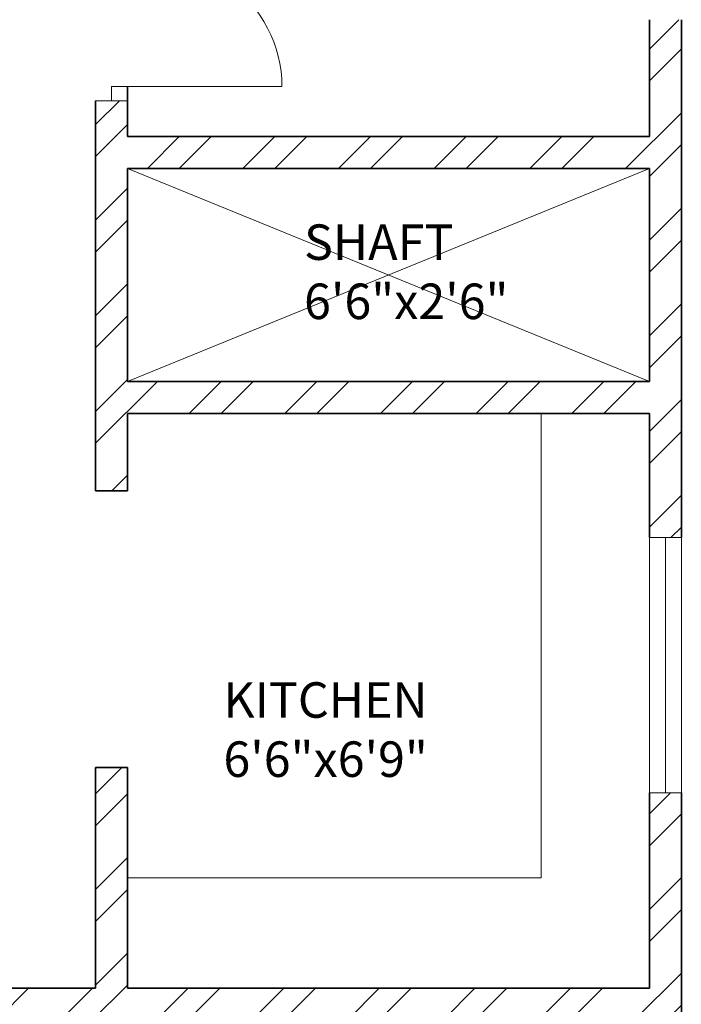
# Model space of a CAD drawing. Units: inches. Extents: x 2168 to 3056, y 1130 to 2629.
# Tile 34 of 42: x 2771 to 2864, y 2079 to 2217. Entities that reach past the tile are written whole.
import ezdxf

# ---------------------------------------------------------------- set-up
doc = ezdxf.new("R2010")
doc.units = ezdxf.units.IN
for name, color, linetype, lineweight in [('A-AREA-IDEN', 7, 'Continuous', 18), ('A-DOOR', 21, 'Continuous', 18), ('A-FLOR-CASE', 71, 'Continuous', 18), ('A-FLOR-OTLN', 7, 'Continuous', 18), ('A-GLAZ', 201, 'Continuous', 18), ('A-WALL', 7, 'Continuous', 35)]:
    doc.layers.add(name, color=color, linetype=linetype, lineweight=lineweight)
doc.layers.add('A-WALL-PATT', color=143, linetype='Continuous', lineweight=13, true_color=0x7aafdf)
doc.styles.get("Standard").update_dxf_attribs({"font": 'arial.ttf'})

msp = doc.modelspace()

# ---------------------------------------------------------------- hatches: boundary and pattern name
at = {"layer": 'A-WALL-PATT'}
h = msp.add_hatch(dxfattribs=at)
h.set_pattern_fill('ANSI32', color=256)
h.paths.add_polyline_path([(2463.8, 2409.39), (2467.39, 2409.39), (2467.39, 2413.89), (2454.77, 2413.89), (2454.77, 2411.64), (2454.77, 2409.39), (2459.3, 2409.39), (2459.3, 2265.39), (2455.64, 2265.39), (2455.64, 2260.89), (2467.35, 2260.89), (2467.35, 2263.14), (2467.35, 2265.39), (2463.8, 2265.39)])
h.paths.add_polyline_path([(2431.6, 2413.89), (2409.65, 2413.89), (2409.65, 2409.39), (2431.6, 2409.39), (2431.6, 2411.64)])
h.paths.add_polyline_path([(2349.65, 2413.89), (2331.8, 2413.89), (2331.8, 2362.67), (2336.3, 2362.67), (2336.3, 2409.39), (2349.65, 2409.39), (2349.65, 2411.64)])
h.paths.add_polyline_path([(2634.15, 2411.64), (2634.15, 2413.89), (2562.29, 2413.89), (2562.29, 2409.39), (2595.8, 2409.39), (2595.8, 2280.31), (2595.83, 2280.31), (2595.83, 2265.39), (2499.91, 2265.39), (2499.91, 2260.89), (2550.8, 2260.89), (2550.8, 2117.31), (2555.3, 2117.31), (2555.3, 2168.08), (2571.93, 2168.08), (2571.93, 2176.89), (2559.8, 2176.89), (2559.8, 2256.39), (2640.8, 2256.39), (2640.8, 2176.89), (2626.43, 2176.89), (2626.43, 2168.08), (2645.3, 2168.08), (2645.3, 2116.64), (2649.8, 2116.64), (2649.8, 2260.89), (2691.25, 2260.89), (2691.25, 2263.14), (2691.25, 2265.39), (2670.65, 2265.39), (2670.65, 2265.36), (2600.3, 2265.36), (2600.3, 2280.26), (2600.3, 2409.39), (2634.15, 2409.39)])
h.paths.add_polyline_path([(2600.3, 2473.89), (2612.84, 2473.89), (2612.84, 2478.39), (2572.64, 2478.39), (2572.64, 2473.89), (2595.8, 2473.89), (2595.8, 2413.89), (2600.3, 2413.89)])
h.paths.add_polyline_path([(2535.8, 2473.89), (2548.64, 2473.89), (2548.64, 2478.39), (2531.4, 2478.39), (2531.4, 2413.89), (2521.6, 2413.89), (2521.6, 2409.39), (2539.24, 2409.39), (2539.24, 2411.64), (2539.24, 2413.89), (2535.8, 2413.89)])
h.paths.add_polyline_path([(2664.8, 2478.39), (2636.84, 2478.39), (2636.84, 2473.89), (2660.3, 2473.89), (2660.3, 2413.89), (2656.17, 2413.89), (2656.17, 2409.39), (2671.68, 2409.39), (2671.68, 2411.64), (2671.68, 2413.89), (2664.8, 2413.89)])
h.paths.add_polyline_path([(2705.94, 2413.89), (2695.68, 2413.89), (2695.68, 2409.39), (2705.94, 2409.39)])
h.paths.add_polyline_path([(2741.35, 2413.89), (2728.73, 2413.89), (2728.73, 2411.64), (2728.73, 2409.39), (2732.3, 2409.39), (2732.3, 2265.39), (2725.73, 2265.39), (2725.73, 2260.89), (2740.92, 2260.89), (2740.92, 2263.14), (2740.92, 2265.39), (2736.8, 2265.39), (2736.8, 2409.39), (2741.35, 2409.39)])
h.paths.add_polyline_path([(2785.65, 2413.89), (2764.55, 2413.89), (2764.49, 2409.39), (2785.65, 2409.39), (2785.65, 2411.64)])
h.paths.add_polyline_path([(2864.3, 2413.89), (2845.65, 2413.89), (2845.65, 2409.39), (2859.8, 2409.39), (2859.8, 2368.43), (2864.3, 2368.43)])
h.paths.add_polyline_path([(2864.3, 2308.43), (2862.05, 2308.43), (2859.8, 2308.43), (2859.8, 2265.39), (2774.48, 2265.39), (2774.48, 2263.14), (2774.48, 2260.89), (2781.8, 2260.89), (2781.8, 2226.65), (2786.3, 2226.65), (2786.3, 2260.89), (2859.8, 2260.89), (2859.8, 2241.35), (2864.3, 2241.35)])
h.paths.add_polyline_path([(2864.3, 2217.35), (2862.05, 2217.35), (2859.8, 2217.35), (2859.8, 2200.89), (2786.3, 2200.89), (2786.3, 2205.93), (2784.05, 2205.93), (2781.8, 2205.93), (2781.8, 2150.97), (2786.3, 2150.97), (2786.3, 2161.89), (2859.8, 2161.89), (2859.8, 2144.42), (2864.3, 2144.42)])
h.paths.add_polyline_path([(2859.8, 2196.39), (2859.8, 2166.39), (2786.3, 2166.39), (2786.3, 2196.39)], flags=16)
h.paths.add_polyline_path([(2864.3, 2108.42), (2862.05, 2108.42), (2859.8, 2108.42), (2859.8, 2080.89), (2786.3, 2080.89), (2786.3, 2111.99), (2781.8, 2111.99), (2781.8, 2080.89), (2649.8, 2080.89), (2649.8, 2086.04), (2647.55, 2086.04), (2645.3, 2086.04), (2645.3, 2071.74), (2649.8, 2071.74), (2649.8, 2076.39), (2781.8, 2076.39), (2781.8, 2041.79), (2786.3, 2041.79), (2786.3, 2076.39), (2859.8, 2076.39), (2859.8, 2058.58), (2864.3, 2058.58)])
h.paths.add_polyline_path([(2864.3, 2022.58), (2859.8, 2022.58), (2859.8, 1992.39), (2786.3, 1992.39), (2786.3, 1999.57), (2781.8, 1999.57), (2781.8, 1848.09), (2784.05, 1848.09), (2786.3, 1848.09), (2786.3, 1851.39), (2859.8, 1851.39), (2859.8, 1838.26), (2864.3, 1838.26)], flags=17)
h.paths.add_polyline_path([(2859.8, 1987.89), (2859.8, 1855.89), (2786.3, 1855.89), (2786.3, 1987.89)], flags=16)
h.paths.add_polyline_path([(2823.05, 1987.89), (2841.42, 1921.89), (2823.05, 1855.89)], flags=0)
h.paths.add_polyline_path([(2864.3, 1814.26), (2859.8, 1814.26), (2859.8, 1791.39), (2786.3, 1791.39), (2786.3, 1825.66), (2784.05, 1825.66), (2781.8, 1825.66), (2781.8, 1791.39), (2720.15, 1791.39), (2720.15, 1791.27), (2649.8, 1791.27), (2649.8, 1806.16), (2649.8, 2038.98), (2647.55, 2038.98), (2645.3, 2038.98), (2645.3, 1783.93), (2649.8, 1783.93), (2649.8, 1786.89), (2781.8, 1786.89), (2781.8, 1746.79), (2786.3, 1746.79), (2786.3, 1786.89), (2859.8, 1786.89), (2859.8, 1770.08), (2864.3, 1770.08)])
h.paths.add_polyline_path([(2864.3, 1734.08), (2862.05, 1734.08), (2859.8, 1734.08), (2859.8, 1705.89), (2786.3, 1705.89), (2786.3, 1714.17), (2781.8, 1714.17), (2781.8, 1660.53), (2786.3, 1660.53), (2786.3, 1666.89), (2859.8, 1666.89), (2859.8, 1648.34), (2864.3, 1648.34)])
h.paths.add_polyline_path([(2786.3, 1701.39), (2859.8, 1701.39), (2859.8, 1671.39), (2786.3, 1671.39)], flags=16)
h.paths.add_polyline_path([(2649.8, 1756.58), (2647.55, 1756.58), (2645.3, 1756.58), (2645.3, 1606.89), (2555.3, 1606.89), (2555.3, 1749.51), (2553.05, 1749.51), (2550.8, 1749.51), (2550.8, 1606.89), (2503.01, 1606.89), (2503.01, 1604.64), (2503.01, 1602.39), (2595.8, 1602.39), (2595.85, 1602.39), (2595.85, 1587.5), (2595.8, 1458.39), (2561.5, 1458.39), (2561.5, 1456.14), (2561.5, 1453.89), (2595.8, 1453.89), (2595.8, 1381.89), (2573.44, 1381.89), (2573.44, 1377.39), (2613.01, 1377.39), (2613.01, 1379.64), (2613.01, 1381.89), (2600.3, 1381.89), (2600.3, 1453.89), (2634.33, 1453.89), (2634.33, 1458.39), (2600.3, 1458.39), (2600.3, 1602.39), (2670.65, 1602.39), (2694.09, 1602.39), (2694.09, 1606.89), (2649.8, 1606.89)])
h.paths.add_polyline_path([(2736.8, 1602.39), (2741.56, 1602.39), (2741.56, 1606.89), (2726.2, 1606.89), (2726.2, 1604.64), (2726.2, 1602.39), (2732.3, 1602.39), (2732.3, 1458.39), (2727.9, 1458.39), (2727.9, 1453.89), (2740.82, 1453.89), (2740.82, 1456.14), (2740.82, 1458.39), (2736.8, 1458.39)])
h.paths.add_polyline_path([(2859.8, 1606.89), (2786.3, 1606.89), (2786.3, 1637.33), (2784.05, 1637.33), (2781.8, 1637.33), (2781.8, 1606.89), (2775.61, 1606.89), (2775.61, 1602.39), (2859.8, 1602.39)])
h.paths.add_polyline_path([(2864.3, 1624.34), (2862.05, 1624.34), (2859.8, 1624.34), (2859.8, 1570.39), (2864.3, 1570.39)])
h.paths.add_polyline_path([(2864.3, 1510.39), (2862.05, 1510.39), (2859.8, 1510.39), (2859.8, 1458.39), (2846.73, 1458.39), (2846.73, 1456.14), (2846.73, 1453.89), (2864.3, 1453.89)])
h.paths.add_polyline_path([(2786.73, 1458.39), (2765.44, 1458.39), (2765.44, 1453.89), (2786.73, 1453.89)])
h.paths.add_polyline_path([(2706, 1458.39), (2695.36, 1458.39), (2695.36, 1453.89), (2706, 1453.89), (2706, 1456.14)])
h.paths.add_polyline_path([(2671.36, 1456.14), (2671.36, 1458.39), (2655.99, 1458.39), (2655.99, 1456.14), (2655.99, 1453.89), (2660.3, 1453.89), (2660.3, 1381.89), (2637.01, 1381.89), (2637.01, 1377.39), (2664.8, 1377.39), (2664.8, 1453.89), (2671.36, 1453.89)], flags=17)
h.paths.add_polyline_path([(2539.83, 1458.39), (2520.24, 1458.39), (2520.24, 1453.89), (2531.3, 1453.89), (2531.3, 1377.39), (2546.45, 1377.39), (2546.45, 1379.64), (2546.45, 1381.89), (2535.8, 1381.89), (2535.8, 1453.89), (2539.83, 1453.89)], flags=17)
h.paths.add_polyline_path([(2496.24, 1458.39), (2489.13, 1458.39), (2489.13, 1453.89), (2496.24, 1453.89), (2496.24, 1456.14)])
h.paths.add_polyline_path([(2467.43, 1456.14), (2467.43, 1458.39), (2463.8, 1458.39), (2463.8, 1602.39), (2468.24, 1602.39), (2468.24, 1605.7), (2468.24, 1606.89), (2454.6, 1606.89), (2454.6, 1602.39), (2459.3, 1602.39), (2459.3, 1458.39), (2454.24, 1458.39), (2454.24, 1453.89), (2467.43, 1453.89)])
h.paths.add_polyline_path([(2431.6, 1456.14), (2431.6, 1458.39), (2411.39, 1458.39), (2411.39, 1453.89), (2431.6, 1453.89)])
h.paths.add_polyline_path([(2351.39, 1458.39), (2336.3, 1458.39), (2336.3, 1490.69), (2334.05, 1490.69), (2331.8, 1490.69), (2331.8, 1453.89), (2351.39, 1453.89), (2351.39, 1456.14)])
h.paths.add_polyline_path([(2336.3, 1629.7), (2331.8, 1629.7), (2331.8, 1552.32), (2336.3, 1552.32), (2336.3, 1602.39), (2406.65, 1602.39), (2423.47, 1602.39), (2423.47, 1606.89), (2418.8, 1606.89), (2418.8, 1643.68), (2416.55, 1643.68), (2414.3, 1643.68), (2414.3, 1606.89), (2336.3, 1606.89)])
h.paths.add_polyline_path([(2418.8, 1714.38), (2414.3, 1714.38), (2414.3, 1705.89), (2336.3, 1705.89), (2336.3, 1731.32), (2334.05, 1731.32), (2331.8, 1731.32), (2331.8, 1653.7), (2334.05, 1653.7), (2336.3, 1653.7), (2336.3, 1666.89), (2414.3, 1666.89), (2414.3, 1663.59), (2418.8, 1663.59)])
h.paths.add_polyline_path([(2336.3, 1701.39), (2414.3, 1701.39), (2414.3, 1671.39), (2336.3, 1671.39)], flags=16)
h.paths.add_polyline_path([(2555.3, 2040.06), (2550.8, 2040.06), (2550.8, 1791.39), (2550.56, 1791.2), (2480.2, 1791.2), (2418.8, 1791.39), (2418.8, 1825.45), (2416.55, 1825.45), (2414.3, 1825.45), (2414.3, 1791.39), (2336.3, 1791.39), (2336.3, 1806.41), (2331.8, 1806.41), (2331.8, 1767.32), (2336.3, 1767.32), (2336.3, 1786.89), (2414.3, 1786.89), (2414.3, 1745.46), (2418.8, 1745.46), (2418.8, 1786.89), (2550.8, 1786.89), (2550.8, 1783.01), (2555.3, 1783.01)])
h.paths.add_polyline_path([(2418.8, 1923.39), (2423.21, 1923.39), (2423.21, 1925.64), (2423.21, 1927.89), (2418.8, 1927.89), (2418.8, 2000.05), (2414.3, 2000.05), (2414.3, 1992.39), (2336.3, 1992.39), (2336.3, 1987.89), (2414.3, 1987.89), (2414.3, 1855.89), (2336.3, 1855.89), (2336.3, 1851.39), (2414.3, 1851.39), (2414.3, 1846.76), (2418.8, 1846.76)], flags=17)
h.paths.add_polyline_path([(2336.3, 2019.29), (2334.05, 2019.29), (2331.8, 2019.29), (2331.8, 1830.41), (2336.3, 1830.41)], flags=17)
h.paths.add_polyline_path([(2550.8, 1927.89), (2453.54, 1927.89), (2453.54, 1925.64), (2453.54, 1923.39), (2550.8, 1923.39)], flags=17)
h.paths.add_polyline_path([(2744.99, 1927.89), (2649.8, 1927.89), (2649.8, 1923.39), (2744.99, 1923.39), (2744.99, 1925.64)], flags=17)
h.paths.add_polyline_path([(2555.3, 2086.46), (2553.05, 2086.46), (2550.8, 2086.46), (2550.8, 2080.89), (2418.8, 2080.89), (2336.3, 2080.89), (2336.3, 2115.4), (2334.05, 2115.4), (2331.8, 2115.4), (2331.8, 2055.29), (2336.3, 2055.29), (2336.3, 2076.39), (2550.8, 2076.39), (2550.8, 2071.54), (2555.3, 2071.54)])
h.paths.add_polyline_path([(2418.8, 2121.39), (2414.3, 2121.39), (2414.3, 2080.89), (2418.8, 2080.89)])
h.paths.add_polyline_path([(2418.8, 2076.39), (2414.3, 2076.39), (2414.3, 2035.12), (2418.8, 2035.12)])
h.paths.add_polyline_path([(2422.87, 2263.14), (2422.87, 2265.39), (2406.65, 2265.39), (2406.65, 2265.36), (2336.3, 2265.36), (2336.3, 2280.25), (2336.3, 2302.67), (2334.05, 2302.67), (2331.8, 2302.67), (2331.8, 2246.85), (2336.3, 2246.85), (2336.3, 2260.89), (2414.3, 2260.89), (2414.3, 2224), (2418.8, 2224), (2418.8, 2260.89), (2422.87, 2260.89)])
h.paths.add_polyline_path([(2418.8, 2204.78), (2416.55, 2204.78), (2414.3, 2204.78), (2414.3, 2200.89), (2336.3, 2200.89), (2336.3, 2220.85), (2331.8, 2220.85), (2331.8, 2151.4), (2336.3, 2151.4), (2336.3, 2161.89), (2414.3, 2161.89), (2414.3, 2153.73), (2418.8, 2153.73)])
h.paths.add_polyline_path([(2414.3, 2196.39), (2414.3, 2166.39), (2336.3, 2166.39), (2336.3, 2196.39)], flags=16)
h.paths.add_polyline_path([(2375.3, 2181.39), (2336.3, 2166.39), (2336.3, 2196.39)], flags=0)
h.paths.add_polyline_path([(2809.6, 2172.34), (2838.8, 2172.34), (2838.8, 2191), (2809.6, 2191)], flags=8)
h.paths.add_polyline_path([(2849.75, 1919.59), (2849.75, 1952.67), (2831.09, 1952.67), (2831.09, 1919.59)], flags=8)
h.paths.add_polyline_path([(2808.87, 1901.97), (2808.87, 1937.85), (2790.15, 1937.85), (2790.15, 1901.97)], flags=8)
h.paths.add_polyline_path([(2806.28, 1671.9), (2835.49, 1671.9), (2835.49, 1690.55), (2806.28, 1690.55)], flags=8)
h.paths.add_polyline_path([(2353.19, 1676.55), (2382.39, 1676.55), (2382.39, 1695.21), (2353.19, 1695.21)], flags=8)
h.paths.add_polyline_path([(2360.08, 1832.31), (2389.24, 1832.31), (2389.24, 1850.97), (2360.08, 1850.97)], flags=25)
h.paths.add_polyline_path([(2354.82, 2167.82), (2384.03, 2167.82), (2384.03, 2186.48), (2354.82, 2186.48)], flags=8)

# ---------------------------------------------------------------- linework, layer by layer
at = {"layer": 'A-DOOR'}
for p, q in [((2784.05, 2205.93), (2784.05, 2207.93)), ((2784.05, 2207.93), (2808.05, 2207.93)), ((2781.8, 2205.93), (2786.3, 2205.93)), ((2786.3, 2205.93), (2784.05, 2205.93))]:
    msp.add_line(p, q, dxfattribs=at)
msp.add_arc((2790.22, 2207.93), 17.83, 360, 110.2649, dxfattribs=at)
at = {"layer": 'A-FLOR-CASE'}
for p, q in [((2844.54, 2096.44), (2844.54, 2161.89)), ((2786.3, 2096.44), (2844.54, 2096.44))]:
    msp.add_line(p, q, dxfattribs=at)
at = {"layer": 'A-FLOR-OTLN'}
for p, q in [((2859.8, 2196.39), (2786.3, 2166.39)), ((2786.3, 2196.39), (2859.8, 2166.39))]:
    msp.add_line(p, q, dxfattribs=at)
at = {"layer": 'A-GLAZ'}
for p, q in [((2862.05, 2144.42), (2859.8, 2144.42)), ((2859.8, 2144.42), (2864.3, 2144.42)), ((2859.8, 2144.42), (2859.8, 2129.86)), ((2862.05, 2108.42), (2862.05, 2144.42)), ((2864.3, 2144.42), (2864.3, 2108.42)), ((2859.8, 2129.86), (2859.8, 2108.42)), ((2859.8, 2108.42), (2864.3, 2108.42)), ((2864.3, 2108.42), (2862.05, 2108.42))]:
    msp.add_line(p, q, dxfattribs=at)
at = {"layer": 'A-WALL'}
for p, q in [((2859.8, 2217.35), (2859.8, 2200.89)), ((2864.3, 2217.35), (2864.3, 2144.42)), ((2786.3, 2207.93), (2786.3, 2200.89)), ((2781.8, 2205.93), (2781.8, 2150.97)), ((2786.3, 2200.89), (2859.8, 2200.89)), ((2786.3, 2196.39), (2859.8, 2196.39)), ((2786.3, 2196.39), (2786.3, 2166.39)), ((2859.8, 2196.39), (2859.8, 2166.39)), ((2786.3, 2166.39), (2859.8, 2166.39)), ((2786.3, 2161.89), (2859.8, 2161.89)), ((2786.3, 2161.89), (2786.3, 2150.97)), ((2859.8, 2161.89), (2859.8, 2144.42)), ((2781.8, 2150.97), (2786.3, 2150.97)), ((2781.8, 2111.99), (2786.3, 2111.99)), ((2781.8, 2111.99), (2781.8, 2080.89)), ((2786.3, 2111.99), (2786.3, 2080.89)), ((2859.8, 2108.42), (2859.8, 2080.89)), ((2864.3, 2108.42), (2864.3, 2058.58)), ((2781.8, 2080.89), (2649.8, 2080.89)), ((2649.8, 2080.89), (2781.8, 2080.89)), ((2786.3, 2080.89), (2859.8, 2080.89))]:
    msp.add_line(p, q, dxfattribs=at)

# ---------------------------------------------------------------- texts
at = {"layer": 'A-AREA-IDEN', "char_height": 5, "attachment_point": 1}
for s, width, insert in [('SHAFT\\P6\'6"x2\'6"', 141.6685, (2811.16, 2188.51)), ('KITCHEN\\P6\'6"x6\'9"', 105.7374, (2799.8, 2124.01))]:
    msp.add_mtext_dynamic_manual_height_columns(s, width=width, gutter_width=12.5, heights=[0], dxfattribs=dict(at, insert=insert))

doc.saveas('drawing.dxf')
